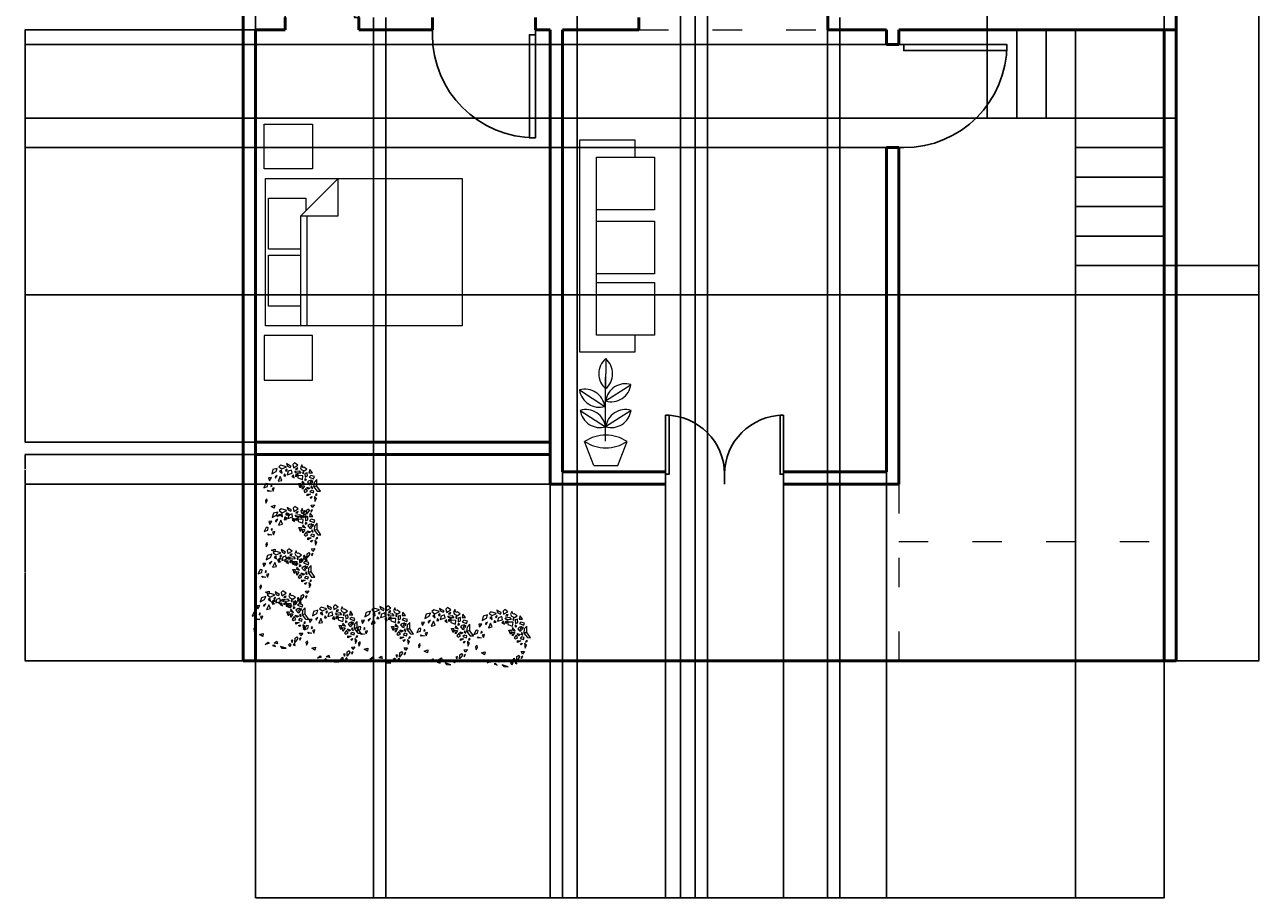
# Model space of a CAD drawing. Units: inches. Extents: x 115999 to 116502, y 188991 to 189729.
# Tile 1 of 5: x 115999 to 116502, y 188991 to 189347. Entities that reach past the tile are written whole.
import ezdxf

# ---------------------------------------------------------------- set-up
doc = ezdxf.new("R2010")
doc.units = ezdxf.units.IN
doc.linetypes.add('ACAD_ISO03W100', pattern=[30, 12, -18])
for name, color, linetype, lineweight in [('A-ANNO-DIMS', 2, 'Continuous', 18), ('A-DOOR', 4, 'Continuous', 25), ('A-FLOR-PRCH', 8, 'ACAD_ISO03W100', 18), ('A-FLOR-STRS', 7, 'Continuous', 25), ('A-FURN', 8, 'Continuous', 18), ('A-WALL', 7, 'Continuous', 50), ('A-WALL-OPEN', 7, 'ACAD_ISO03W100', 18), ('L-PLNT', 3, 'Continuous', 13)]:
    doc.layers.add(name, color=color, linetype=linetype, lineweight=lineweight)
doc.styles.get("Standard").update_dxf_attribs({"font": 'arial.ttf'})
doc.dimstyles.get("Standard").update_dxf_attribs({"dimtxt": 0.18, "dimasz": 0.18, "dimexe": 0.18, "dimexo": 0.0625, "dimgap": 0.09, "dimtad": 0, "dimtih": 1, "dimtoh": 1, "dimdec": 4, "dimzin": 0, "dimdsep": 46, "dimtxsty": 'Standard', "dimcen": 0.09, "dimadec": 0, "dimazin": 0, "dimtfac": 1, "dimtdec": 4, "dimtofl": 0, "dimtmove": 0, "dimatfit": 3, "dimfxl": 1, "dimtolj": 1, "dimtzin": 0, "dimarcsym": 0})

# ---------------------------------------------------------------- blocks, each defined once
blk = doc.blocks.new('*U3')
for p, q in [((0, 0), (0, -5)), ((30, 0), (30, -5))]:
    blk.add_line(p, q)
blk.add_lwpolyline([(0, 0), (0, 30), (1.75, 30), (1.75, 0)], close=True)
blk.add_arc((0, 0), 30, 0, 90)
blk = doc.blocks.new('Bed - Queen')
for p, q in [((0, -80.00003), (0, 0)), ((0, 0), (59.99999, 0)), ((59.99999, 0), (59.99999, -80.00003)), ((7.99999, -1.2), (28.79998, -1.2)), ((7.99999, -14.4), (7.99999, -1.2)), ((28.79998, -1.2), (28.79998, -14.4)), ((31.19999, -1.2), (51.99999, -1.2)), ((31.19999, -14.4), (31.19999, -1.2)), ((51.99999, -1.2), (51.99999, -16.4)), ((0, -14.4), (44.8, -14.4)), ((59.99999, -29.6), (44.8, -14.4)), ((44.8, -14.4), (44.8, -29.6)), ((44.8, -16.8), (0, -16.8)), ((51.99999, -16.4), (46.79936, -16.4)), ((44.8, -29.6), (59.99999, -29.6)), ((59.99999, -80.00003), (0, -80.00003))]:
    blk.add_line(p, q)
blk = doc.blocks.new('*U9')
for points in [[(-4.43, 11.05), (-5.18, 10.36), (-3.96, 9.49), (-2.07, 10.36)], [(-2, 11.66), (-1.6, 10.62), (-0.52, 10.1), (-0.18, 10.62), (-0.79, 10.96)], [(1.24, 12), (0.56, 11.31), (0.76, 10.01), (2.52, 11.05)], [(4.14, 11.14), (3.6, 10.01), (4, 9.23), (5.22, 8.71), (6.3, 9.41), (5.08, 10.19), (4.61, 10.01)], [(-8.14, 6.03), (-9.36, 5.95), (-9.02, 4.73)], [(-5.78, 9.75), (-7.54, 9.23), (-8.01, 7.5), (-6.26, 8.45)], [(-5.78, 6.81), (-6.66, 6.21), (-6.52, 5.69)], [(-4.57, 6.38), (-5.45, 4.47), (-3.89, 4.82)], [(-4.84, 8.63), (-3.83, 7.85), (-4.03, 8.97)], [(-2.88, 7.5), (-3.15, 6.64), (-2.27, 6.72)], [(-1.94, 9.49), (-2.48, 8.97), (-2.27, 8.54), (-1.8, 9.06)], [(0.02, 9.06), (-1.33, 8.54), (-1.73, 7.16), (0.29, 7.76)], [(0.76, 7.16), (0.09, 6.46), (1.1, 5.95)], [(1.37, 8.54), (3.13, 8.8), (3.8, 7.85), (1.91, 7.76)], [(2.59, 9.93), (1.84, 9.75), (1.64, 9.23), (2.32, 9.41)], [(1.71, 6.29), (1.71, 7.07), (2.65, 7.5), (2.11, 6.9)], [(2.52, 6.81), (2.52, 5.86), (4.41, 5.17), (4.61, 6.72)], [(4.61, 8.28), (4.54, 7.76), (4.95, 7.59), (4.95, 8.28)], [(5.49, 5.51), (5.42, 4.82), (6.16, 5.08)], [(6.43, 7.94), (5.49, 7.68), (5.56, 6.21), (6.5, 6.64)], [(7.45, 9.32), (7.11, 7.94), (8.52, 7.94)], [(7.85, 6.81), (7.18, 6.21), (9, 5.51), (9.33, 6.38)], [(10.28, 5.17), (9.2, 4.04), (9, 2.31), (10.48, 0.49), (11.76, 0.41), (10.35, 2.48), (9.33, 2.4), (10.28, 2.83)], [(-11.32, 1.79), (-9.83, 2.31), (-9.63, 3.44), (-10.44, 3.52)], [(-8.21, 0.41), (-9.43, 0.32), (-9.83, 0.84)], [(-8.21, 3.09), (-8.48, 2.31), (-7.87, 2.57)], [(-7, 1.79), (-7.94, 1.53), (-7.47, 0.49)], [(3.53, 1.88), (2.86, 3.52), (3.8, 3.52)], [(4.41, 4.56), (4.27, 3.7), (5.49, 3.26)], [(4.27, 2.74), (5.29, 2.66), (4.41, 1.27)], [(5.83, 1.53), (5.02, 0.41), (5.49, -0.02), (6.5, 0.41)], [(7.51, 1.71), (6.91, 1.27), (6.23, 2.14)], [(8.12, 4.99), (7.11, 4.65), (6.5, 4.13), (7.38, 3.09), (8.12, 3.52), (7.65, 3.87)], [(8.12, 0.75), (7.51, 0.15), (8.93, -0.28), (9.13, 0.49)], [(8.19, 2.57), (7.92, 2.05), (8.66, 1.53)], [(8.73, 4.73), (8.19, 4.56), (8.39, 3.87), (8.59, 4.04)], [(-10.03, -2.71), (-10.64, -3.31), (-10.44, -4.44), (-9.9, -3.49)], [(7.78, -0.8), (6.43, -1.5), (6.43, -0.72)], [(8.32, -1.75), (7.98, -2.53), (7.58, -2.1)], [(9.33, -1.75), (9.54, -3.74), (10.14, -2.53)], [(10.08, -0.63), (9.74, -1.32), (10.48, -0.89)], [(-8.28, -5.73), (-6.79, -5.3), (-7, -6.51)], [(-4.84, -8.85), (-4.43, -9.45), (-5.99, -9.8)], [(-2.34, -9.2), (-1.26, -8.5), (-0.99, -9.54)], [(4.07, -9.45), (3.53, -9.97), (4.07, -10.58), (4.61, -9.89)], [(5.29, -7.98), (4.61, -8.16), (5.02, -8.94)], [(6.03, -9.45), (5.42, -9.97), (6.16, -10.15)], [(6.1, -8.94), (6.16, -7.21), (6.91, -6.69), (7.24, -7.38)], [(8.05, -8.07), (8.59, -7.12), (7.92, -7.55)], [(9.33, -5.13), (8.46, -6.25), (7.98, -5.22)], [(-2.54, -10.06), (-3.02, -10.23), (-1.8, -10.67)], [(0.22, -10.58), (0.83, -11.27), (2.59, -11.36)]]:
    blk.add_lwpolyline(points, close=True)
blk = doc.blocks.new('SOFA-3-SEAT')
for points in [[(22.47, 6.88), (22.47, 0), (0, 0), (0, 86.44), (22.47, 86.44), (22.47, 79.43)], [(29.89, 6.88), (6.84, 6.88), (6.84, 79.43), (29.89, 79.43)]]:
    blk.add_lwpolyline(points)
for points in [[(30.42, 57.99), (6.84, 57.99), (6.84, 79.43), (30.42, 79.43)], [(30.42, 31.86), (6.84, 31.86), (6.84, 53.3), (30.42, 53.3)], [(30.42, 6.88), (6.84, 6.88), (6.84, 28.33), (30.42, 28.33)]]:
    blk.add_lwpolyline(points, close=True)
blk = doc.blocks.new('TABLE-NIGHTSTAND')
blk.add_lwpolyline([(0, 18.2), (19.71, 18.2), (19.71, 0), (0, 0)], close=True)
blk = doc.blocks.new('PLANT-LEAF')
blk.add_line((0, 0.31), (10.34, 7.03))
for centre, start, end in [((8.1, -0.84), 74.1664, 171.9129), ((2.23, 8.18), 254.1664, 351.9129)]:
    blk.add_arc(centre, 8.18, start, end)
blk = doc.blocks.new('*D33')
at = {"layer": 'A-ANNO-DIMS', "color": 0, "lineweight": -2, "transparency": 16777216}
for p, q in [((116088.06, 189088.01), (116088.06, 189728.73)), ((116088.24, 189728.55), (116277.77, 189728.55)), ((116467.88, 189728.55), (116278.35, 189728.55)), ((116468.06, 189088.01), (116468.06, 189728.73))]:
    blk.add_line(p, q, dxfattribs=at)
at = {"layer": 'A-ANNO-DIMS', "color": 0, "transparency": 16777216}
for points in [[(116088.24, 189728.58), (116088.24, 189728.52), (116088.06, 189728.55)], [(116467.88, 189728.58), (116467.88, 189728.52), (116468.06, 189728.55)]]:
    blk.add_solid(points, dxfattribs=at)
at = {"layer": 'Defpoints', "color": 0, "transparency": 16777216}
for p in [(116468.06, 189728.55), (116088.06, 189087.95), (116468.06, 189087.95)]:
    blk.add_point(p, dxfattribs=at)
at = {"layer": 'A-ANNO-DIMS', "color": 0, "transparency": 16777216, "insert": (116278.06, 189728.55), "char_height": 0.18, "attachment_point": 5}
blk.add_mtext('\\A1;380', dxfattribs=at)
blk = doc.blocks.new('*D34')
at = {"layer": 'A-ANNO-DIMS', "color": 0, "lineweight": -2, "transparency": 16777216}
for p, q in [((116468.13, 189694.95), (116501.84, 189694.95)), ((116501.66, 189694.77), (116501.66, 189391.63)), ((116501.66, 189088.13), (116501.66, 189391.27)), ((116468.13, 189087.95), (116501.84, 189087.95))]:
    blk.add_line(p, q, dxfattribs=at)
at = {"layer": 'A-ANNO-DIMS', "color": 0, "transparency": 16777216}
for points in [[(116501.63, 189694.77), (116501.69, 189694.77), (116501.66, 189694.95)], [(116501.63, 189088.13), (116501.69, 189088.13), (116501.66, 189087.95)]]:
    blk.add_solid(points, dxfattribs=at)
at = {"layer": 'Defpoints', "color": 0, "transparency": 16777216}
for p in [(116468.06, 189694.95), (116501.66, 189694.95), (116468.06, 189087.95)]:
    blk.add_point(p, dxfattribs=at)
at = {"layer": 'A-ANNO-DIMS', "color": 0, "transparency": 16777216, "insert": (116501.66, 189391.45), "char_height": 0.18, "attachment_point": 5}
blk.add_mtext('\\A1;607', dxfattribs=at)
blk = doc.blocks.new('*D40')
at = {"layer": 'A-ANNO-DIMS', "color": 0, "lineweight": -2, "transparency": 16777216}
for p, q in [((116093, 189344.95), (115999.04, 189344.95)), ((115999.22, 189344.77), (115999.22, 189261.13)), ((115999.22, 189177.13), (115999.22, 189260.77)), ((116093, 189176.95), (115999.04, 189176.95))]:
    blk.add_line(p, q, dxfattribs=at)
at = {"layer": 'A-ANNO-DIMS', "color": 0, "transparency": 16777216}
for points in [[(115999.19, 189344.77), (115999.25, 189344.77), (115999.22, 189344.95)], [(115999.19, 189177.13), (115999.25, 189177.13), (115999.22, 189176.95)]]:
    blk.add_solid(points, dxfattribs=at)
at = {"layer": 'Defpoints', "color": 0, "transparency": 16777216}
for p in [(116093.06, 189344.95), (115999.22, 189176.95), (116093.06, 189176.95)]:
    blk.add_point(p, dxfattribs=at)
at = {"layer": 'A-ANNO-DIMS', "color": 0, "transparency": 16777216, "insert": (115999.22, 189260.95), "char_height": 0.18, "attachment_point": 5}
blk.add_mtext('\\A1;168', dxfattribs=at)
blk = doc.blocks.new('*D43')
at = {"layer": 'A-ANNO-DIMS', "color": 0, "lineweight": -2, "transparency": 16777216}
for p, q in [((116093.06, 189624.88), (116093.06, 188991.26)), ((116272.06, 189624.88), (116272.06, 188991.26)), ((116093.24, 188991.44), (116182.28, 188991.44)), ((116271.88, 188991.44), (116182.84, 188991.44))]:
    blk.add_line(p, q, dxfattribs=at)
at = {"layer": 'A-ANNO-DIMS', "color": 0, "transparency": 16777216}
for points in [[(116093.24, 188991.47), (116093.24, 188991.41), (116093.06, 188991.44)], [(116271.88, 188991.47), (116271.88, 188991.41), (116272.06, 188991.44)]]:
    blk.add_solid(points, dxfattribs=at)
at = {"layer": 'Defpoints', "color": 0, "transparency": 16777216}
for p in [(116093.06, 189624.95), (116272.06, 189624.95), (116272.06, 188991.44)]:
    blk.add_point(p, dxfattribs=at)
at = {"layer": 'A-ANNO-DIMS', "color": 0, "transparency": 16777216, "insert": (116182.56, 188991.44), "char_height": 0.18, "attachment_point": 5}
blk.add_mtext('\\A1;179', dxfattribs=at)
blk = doc.blocks.new('*D44')
at = {"layer": 'A-ANNO-DIMS', "color": 0, "lineweight": -2, "transparency": 16777216}
for p, q in [((116277.06, 189624.88), (116277.06, 188991.26)), ((116463.06, 189624.88), (116463.06, 188991.26)), ((116277.24, 188991.44), (116369.78, 188991.44)), ((116462.88, 188991.44), (116370.34, 188991.44))]:
    blk.add_line(p, q, dxfattribs=at)
at = {"layer": 'A-ANNO-DIMS', "color": 0, "transparency": 16777216}
for points in [[(116277.24, 188991.47), (116277.24, 188991.41), (116277.06, 188991.44)], [(116462.88, 188991.47), (116462.88, 188991.41), (116463.06, 188991.44)]]:
    blk.add_solid(points, dxfattribs=at)
at = {"layer": 'Defpoints', "color": 0, "transparency": 16777216}
for p in [(116277.06, 189624.95), (116463.06, 189624.95), (116463.06, 188991.44)]:
    blk.add_point(p, dxfattribs=at)
at = {"layer": 'A-ANNO-DIMS', "color": 0, "transparency": 16777216, "insert": (116370.06, 188991.44), "char_height": 0.18, "attachment_point": 5}
blk.add_mtext('\\A1;186', dxfattribs=at)
blk = doc.blocks.new('*D45')
at = {"layer": 'A-ANNO-DIMS', "color": 0, "lineweight": -2, "transparency": 16777216}
for p, q in [((116272.06, 189624.88), (116272.06, 188991.26)), ((116277.06, 189624.88), (116277.06, 188991.26)), ((116272.24, 188991.44), (116274.41, 188991.44)), ((116276.88, 188991.44), (116274.71, 188991.44))]:
    blk.add_line(p, q, dxfattribs=at)
at = {"layer": 'A-ANNO-DIMS', "color": 0, "transparency": 16777216}
for points in [[(116272.24, 188991.47), (116272.24, 188991.41), (116272.06, 188991.44)], [(116276.88, 188991.47), (116276.88, 188991.41), (116277.06, 188991.44)]]:
    blk.add_solid(points, dxfattribs=at)
at = {"layer": 'Defpoints', "color": 0, "transparency": 16777216}
for p in [(116272.06, 189624.95), (116277.06, 189624.95), (116277.06, 188991.44)]:
    blk.add_point(p, dxfattribs=at)
at = {"layer": 'A-ANNO-DIMS', "color": 0, "transparency": 16777216, "insert": (116274.56, 188991.44), "char_height": 0.18, "attachment_point": 5}
blk.add_mtext('\\A1;5', dxfattribs=at)
blk = doc.blocks.new('*D46')
at = {"layer": 'A-ANNO-DIMS', "color": 0, "lineweight": -2, "transparency": 16777216}
for p, q in [((116224.06, 189486.88), (116224.06, 188991.26)), ((116266.06, 189486.88), (116266.06, 188991.26)), ((116224.24, 188991.44), (116244.84, 188991.44)), ((116265.88, 188991.44), (116245.28, 188991.44))]:
    blk.add_line(p, q, dxfattribs=at)
at = {"layer": 'A-ANNO-DIMS', "color": 0, "transparency": 16777216}
for points in [[(116224.24, 188991.47), (116224.24, 188991.41), (116224.06, 188991.44)], [(116265.88, 188991.47), (116265.88, 188991.41), (116266.06, 188991.44)]]:
    blk.add_solid(points, dxfattribs=at)
at = {"layer": 'Defpoints', "color": 0, "transparency": 16777216}
for p in [(116224.06, 189486.95), (116266.06, 189486.95), (116266.06, 188991.44)]:
    blk.add_point(p, dxfattribs=at)
at = {"layer": 'A-ANNO-DIMS', "color": 0, "transparency": 16777216, "insert": (116245.06, 188991.44), "char_height": 0.18, "attachment_point": 5}
blk.add_mtext('\\A1;42', dxfattribs=at)
blk = doc.blocks.new('*D47')
at = {"layer": 'A-ANNO-DIMS', "color": 0, "lineweight": -2, "transparency": 16777216}
for p, q in [((116266.063078, 189486.884428), (116266.063078, 188991.259265)), ((116272.063078, 189486.884428), (116272.063078, 188991.259265)), ((116266.243078, 188991.439265), (116268.913651, 188991.439265)), ((116271.883078, 188991.439265), (116269.212505, 188991.439265))]:
    blk.add_line(p, q, dxfattribs=at)
at = {"layer": 'A-ANNO-DIMS', "color": 0, "transparency": 16777216}
for points in [[(116266.243078, 188991.469265), (116266.243078, 188991.409265), (116266.063078, 188991.439265)], [(116271.883078, 188991.469265), (116271.883078, 188991.409265), (116272.063078, 188991.439265)]]:
    blk.add_solid(points, dxfattribs=at)
at = {"layer": 'Defpoints', "color": 0, "transparency": 16777216}
for p in [(116266.063078, 189486.946928), (116272.063078, 189486.946928), (116272.063078, 188991.439265)]:
    blk.add_point(p, dxfattribs=at)
at = {"layer": 'A-ANNO-DIMS', "color": 0, "transparency": 16777216, "insert": (116269.063078, 188991.439265), "char_height": 0.18, "attachment_point": 5}
blk.add_mtext('\\A1;6', dxfattribs=at)
blk = doc.blocks.new('*D49')
at = {"layer": 'A-ANNO-DIMS', "color": 0, "lineweight": -2, "transparency": 16777216}
for p, q in [((116331.06, 189349.88), (116331.06, 188991.26)), ((116463.06, 189349.88), (116463.06, 188991.26)), ((116331.24, 188991.44), (116396.78, 188991.44)), ((116462.88, 188991.44), (116397.34, 188991.44))]:
    blk.add_line(p, q, dxfattribs=at)
at = {"layer": 'A-ANNO-DIMS', "color": 0, "transparency": 16777216}
for points in [[(116331.24, 188991.47), (116331.24, 188991.41), (116331.06, 188991.44)], [(116462.88, 188991.47), (116462.88, 188991.41), (116463.06, 188991.44)]]:
    blk.add_solid(points, dxfattribs=at)
at = {"layer": 'Defpoints', "color": 0, "transparency": 16777216}
for p in [(116331.06, 189349.95), (116463.06, 189349.95), (116463.06, 188991.44)]:
    blk.add_point(p, dxfattribs=at)
at = {"layer": 'A-ANNO-DIMS', "color": 0, "transparency": 16777216, "insert": (116397.06, 188991.44), "char_height": 0.18, "attachment_point": 5}
blk.add_mtext('\\A1;132', dxfattribs=at)
blk = doc.blocks.new('*D50')
at = {"layer": 'A-ANNO-DIMS', "color": 0, "lineweight": -2, "transparency": 16777216}
for p, q in [((116146.06, 189349.88), (116146.06, 188991.26)), ((116326.06, 189349.88), (116326.06, 188991.26)), ((116146.24, 188991.44), (116235.78, 188991.44)), ((116325.88, 188991.44), (116236.34, 188991.44))]:
    blk.add_line(p, q, dxfattribs=at)
at = {"layer": 'A-ANNO-DIMS', "color": 0, "transparency": 16777216}
for points in [[(116146.24, 188991.47), (116146.24, 188991.41), (116146.06, 188991.44)], [(116325.88, 188991.47), (116325.88, 188991.41), (116326.06, 188991.44)]]:
    blk.add_solid(points, dxfattribs=at)
at = {"layer": 'Defpoints', "color": 0, "transparency": 16777216}
for p in [(116146.06, 189349.95), (116326.06, 189349.95), (116326.06, 188991.44)]:
    blk.add_point(p, dxfattribs=at)
at = {"layer": 'A-ANNO-DIMS', "color": 0, "transparency": 16777216, "insert": (116236.06, 188991.44), "char_height": 0.18, "attachment_point": 5}
blk.add_mtext('\\A1;180', dxfattribs=at)
blk = doc.blocks.new('*D51')
at = {"layer": 'A-ANNO-DIMS', "color": 0, "lineweight": -2, "transparency": 16777216}
for p, q in [((116093.06, 189349.88), (116093.06, 188991.26)), ((116141.06, 189349.88), (116141.06, 188991.26)), ((116093.24, 188991.44), (116116.84, 188991.44)), ((116140.88, 188991.44), (116117.29, 188991.44))]:
    blk.add_line(p, q, dxfattribs=at)
at = {"layer": 'A-ANNO-DIMS', "color": 0, "transparency": 16777216}
for points in [[(116093.24, 188991.47), (116093.24, 188991.41), (116093.06, 188991.44)], [(116140.88, 188991.47), (116140.88, 188991.41), (116141.06, 188991.44)]]:
    blk.add_solid(points, dxfattribs=at)
at = {"layer": 'Defpoints', "color": 0, "transparency": 16777216}
for p in [(116093.06, 189349.95), (116141.06, 189349.95), (116141.06, 188991.44)]:
    blk.add_point(p, dxfattribs=at)
at = {"layer": 'A-ANNO-DIMS', "color": 0, "transparency": 16777216, "insert": (116117.06, 188991.44), "char_height": 0.18, "attachment_point": 5}
blk.add_mtext('\\A1;48', dxfattribs=at)
blk = doc.blocks.new('*D56')
at = {"layer": 'A-ANNO-DIMS', "color": 0, "lineweight": -2, "transparency": 16777216}
for p, q in [((116093.06, 189176.88), (116093.06, 188991.26)), ((116213.06, 189176.88), (116213.06, 188991.26)), ((116093.24, 188991.44), (116152.78, 188991.44)), ((116212.88, 188991.44), (116153.34, 188991.44))]:
    blk.add_line(p, q, dxfattribs=at)
at = {"layer": 'A-ANNO-DIMS', "color": 0, "transparency": 16777216}
for points in [[(116093.24, 188991.47), (116093.24, 188991.41), (116093.06, 188991.44)], [(116212.88, 188991.47), (116212.88, 188991.41), (116213.06, 188991.44)]]:
    blk.add_solid(points, dxfattribs=at)
at = {"layer": 'Defpoints', "color": 0, "transparency": 16777216}
for p in [(116093.06, 189176.95), (116213.06, 189176.95), (116213.06, 188991.44)]:
    blk.add_point(p, dxfattribs=at)
at = {"layer": 'A-ANNO-DIMS', "color": 0, "transparency": 16777216, "insert": (116153.06, 188991.44), "char_height": 0.18, "attachment_point": 5}
blk.add_mtext('\\A1;120', dxfattribs=at)
blk = doc.blocks.new('*D57')
at = {"layer": 'A-ANNO-DIMS', "color": 0, "lineweight": -2, "transparency": 16777216}
for p, q in [((116218.06, 189164.88), (116218.06, 188991.26)), ((116260.06, 189164.88), (116260.06, 188991.26)), ((116218.24, 188991.44), (116238.84, 188991.44)), ((116259.88, 188991.44), (116239.28, 188991.44))]:
    blk.add_line(p, q, dxfattribs=at)
at = {"layer": 'A-ANNO-DIMS', "color": 0, "transparency": 16777216}
for points in [[(116218.24, 188991.47), (116218.24, 188991.41), (116218.06, 188991.44)], [(116259.88, 188991.47), (116259.88, 188991.41), (116260.06, 188991.44)]]:
    blk.add_solid(points, dxfattribs=at)
at = {"layer": 'Defpoints', "color": 0, "transparency": 16777216}
for p in [(116218.06, 189164.95), (116260.06, 189164.95), (116260.06, 188991.44)]:
    blk.add_point(p, dxfattribs=at)
at = {"layer": 'A-ANNO-DIMS', "color": 0, "transparency": 16777216, "insert": (116239.06, 188991.44), "char_height": 0.18, "attachment_point": 5}
blk.add_mtext('\\A1;42', dxfattribs=at)
blk = doc.blocks.new('*D58')
at = {"layer": 'A-ANNO-DIMS', "color": 0, "lineweight": -2, "transparency": 16777216}
for p, q in [((116260.06, 189164.88), (116260.06, 188991.26)), ((116308.06, 189164.88), (116308.06, 188991.26)), ((116260.24, 188991.44), (116283.84, 188991.44)), ((116307.88, 188991.44), (116284.29, 188991.44))]:
    blk.add_line(p, q, dxfattribs=at)
at = {"layer": 'A-ANNO-DIMS', "color": 0, "transparency": 16777216}
for points in [[(116260.24, 188991.47), (116260.24, 188991.41), (116260.06, 188991.44)], [(116307.88, 188991.47), (116307.88, 188991.41), (116308.06, 188991.44)]]:
    blk.add_solid(points, dxfattribs=at)
at = {"layer": 'Defpoints', "color": 0, "transparency": 16777216}
for p in [(116260.06, 189164.95), (116308.06, 189164.95), (116308.06, 188991.44)]:
    blk.add_point(p, dxfattribs=at)
at = {"layer": 'A-ANNO-DIMS', "color": 0, "transparency": 16777216, "insert": (116284.06, 188991.44), "char_height": 0.18, "attachment_point": 5}
blk.add_mtext('\\A1;48', dxfattribs=at)
blk = doc.blocks.new('*D59')
at = {"layer": 'A-ANNO-DIMS', "color": 0, "lineweight": -2, "transparency": 16777216}
for p, q in [((116308.06, 189164.88), (116308.06, 188991.26)), ((116350.06, 189164.88), (116350.06, 188991.26)), ((116308.24, 188991.44), (116328.84, 188991.44)), ((116349.88, 188991.44), (116329.28, 188991.44))]:
    blk.add_line(p, q, dxfattribs=at)
at = {"layer": 'A-ANNO-DIMS', "color": 0, "transparency": 16777216}
for points in [[(116308.24, 188991.47), (116308.24, 188991.41), (116308.06, 188991.44)], [(116349.88, 188991.47), (116349.88, 188991.41), (116350.06, 188991.44)]]:
    blk.add_solid(points, dxfattribs=at)
at = {"layer": 'Defpoints', "color": 0, "transparency": 16777216}
for p in [(116308.06, 189164.95), (116350.06, 189164.95), (116350.06, 188991.44)]:
    blk.add_point(p, dxfattribs=at)
at = {"layer": 'A-ANNO-DIMS', "color": 0, "transparency": 16777216, "insert": (116329.06, 188991.44), "char_height": 0.18, "attachment_point": 5}
blk.add_mtext('\\A1;42', dxfattribs=at)
blk = doc.blocks.new('*D60')
at = {"layer": 'A-ANNO-DIMS', "color": 0, "lineweight": -2, "transparency": 16777216}
for p, q in [((116213, 189159.95), (115999.04, 189159.95)), ((115999.22, 189159.77), (115999.22, 189124.13)), ((115999.22, 189088.13), (115999.22, 189123.77)), ((116088, 189087.95), (115999.04, 189087.95))]:
    blk.add_line(p, q, dxfattribs=at)
at = {"layer": 'A-ANNO-DIMS', "color": 0, "transparency": 16777216}
for points in [[(115999.19, 189159.77), (115999.25, 189159.77), (115999.22, 189159.95)], [(115999.19, 189088.13), (115999.25, 189088.13), (115999.22, 189087.95)]]:
    blk.add_solid(points, dxfattribs=at)
at = {"layer": 'Defpoints', "color": 0, "transparency": 16777216}
for p in [(116213.06, 189159.95), (115999.22, 189087.95), (116088.06, 189087.95)]:
    blk.add_point(p, dxfattribs=at)
at = {"layer": 'A-ANNO-DIMS', "color": 0, "transparency": 16777216, "insert": (115999.22, 189123.95), "char_height": 0.18, "attachment_point": 5}
blk.add_mtext('\\A1;72', dxfattribs=at)
blk = doc.blocks.new('*D61')
at = {"layer": 'A-ANNO-DIMS', "color": 0, "lineweight": -2, "transparency": 16777216}
for p, q in [((116213, 189171.95), (115999.04, 189171.95)), ((115999.22, 189171.77), (115999.22, 189166.13)), ((115999.22, 189160.13), (115999.22, 189165.77)), ((116213, 189159.95), (115999.04, 189159.95))]:
    blk.add_line(p, q, dxfattribs=at)
at = {"layer": 'A-ANNO-DIMS', "color": 0, "transparency": 16777216}
for points in [[(115999.19, 189171.77), (115999.25, 189171.77), (115999.22, 189171.95)], [(115999.19, 189160.13), (115999.25, 189160.13), (115999.22, 189159.95)]]:
    blk.add_solid(points, dxfattribs=at)
at = {"layer": 'Defpoints', "color": 0, "transparency": 16777216}
for p in [(116213.06, 189171.95), (115999.22, 189159.95), (116213.06, 189159.95)]:
    blk.add_point(p, dxfattribs=at)
at = {"layer": 'A-ANNO-DIMS', "color": 0, "transparency": 16777216, "insert": (115999.22, 189165.95), "char_height": 0.18, "attachment_point": 5}
blk.add_mtext('\\A1;12', dxfattribs=at)
blk = doc.blocks.new('*D62')
at = {"layer": 'A-ANNO-DIMS', "color": 0, "lineweight": -2, "transparency": 16777216}
for p, q in [((116427.06, 189236.88), (116427.06, 188991.26)), ((116463.06, 189236.88), (116463.06, 188991.26)), ((116427.24, 188991.44), (116444.84, 188991.44)), ((116462.88, 188991.44), (116445.28, 188991.44))]:
    blk.add_line(p, q, dxfattribs=at)
at = {"layer": 'A-ANNO-DIMS', "color": 0, "transparency": 16777216}
for points in [[(116427.24, 188991.47), (116427.24, 188991.41), (116427.06, 188991.44)], [(116462.88, 188991.47), (116462.88, 188991.41), (116463.06, 188991.44)]]:
    blk.add_solid(points, dxfattribs=at)
at = {"layer": 'Defpoints', "color": 0, "transparency": 16777216}
for p in [(116427.06, 189236.95), (116463.06, 189236.95), (116463.06, 188991.44)]:
    blk.add_point(p, dxfattribs=at)
at = {"layer": 'A-ANNO-DIMS', "color": 0, "transparency": 16777216, "insert": (116445.06, 188991.44), "char_height": 0.18, "attachment_point": 5}
blk.add_mtext('\\A1;36', dxfattribs=at)
blk = doc.blocks.new('*D63')
at = {"layer": 'A-ANNO-DIMS', "color": 0, "lineweight": -2, "transparency": 16777216}
for p, q in [((116415, 189308.95), (115999.04, 189308.95)), ((115999.22, 189308.77), (115999.22, 189273.13)), ((115999.22, 189237.13), (115999.22, 189272.77)), ((116427, 189236.95), (115999.04, 189236.95))]:
    blk.add_line(p, q, dxfattribs=at)
at = {"layer": 'A-ANNO-DIMS', "color": 0, "transparency": 16777216}
for points in [[(115999.19, 189308.77), (115999.25, 189308.77), (115999.22, 189308.95)], [(115999.19, 189237.13), (115999.25, 189237.13), (115999.22, 189236.95)]]:
    blk.add_solid(points, dxfattribs=at)
at = {"layer": 'Defpoints', "color": 0, "transparency": 16777216}
for p in [(116415.06, 189308.95), (115999.22, 189236.95), (116427.06, 189236.95)]:
    blk.add_point(p, dxfattribs=at)
at = {"layer": 'A-ANNO-DIMS', "color": 0, "transparency": 16777216, "insert": (115999.22, 189272.95), "char_height": 0.18, "attachment_point": 5}
blk.add_mtext('\\A1;72', dxfattribs=at)
blk = doc.blocks.new('*D64')
at = {"layer": 'A-ANNO-DIMS', "color": 0, "lineweight": -2, "transparency": 16777216}
for p, q in [((116463.13, 189248.95), (116501.84, 189248.95)), ((116501.66, 189248.77), (116501.66, 189243.13)), ((116501.66, 189237.13), (116501.66, 189242.77)), ((116463.13, 189236.95), (116501.84, 189236.95))]:
    blk.add_line(p, q, dxfattribs=at)
at = {"layer": 'A-ANNO-DIMS', "color": 0, "transparency": 16777216}
for points in [[(116501.63, 189248.77), (116501.69, 189248.77), (116501.66, 189248.95)], [(116501.63, 189237.13), (116501.69, 189237.13), (116501.66, 189236.95)]]:
    blk.add_solid(points, dxfattribs=at)
at = {"layer": 'Defpoints', "color": 0, "transparency": 16777216}
for p in [(116463.06, 189248.95), (116463.06, 189236.95), (116501.66, 189236.95)]:
    blk.add_point(p, dxfattribs=at)
at = {"layer": 'A-ANNO-DIMS', "color": 0, "transparency": 16777216, "insert": (116501.66, 189242.95), "char_height": 0.18, "attachment_point": 5}
blk.add_mtext('\\A1;12', dxfattribs=at)
blk = doc.blocks.new('*D65')
at = {"layer": 'A-ANNO-DIMS', "color": 0, "lineweight": -2, "transparency": 16777216}
for p, q in [((116391.06, 189309.01), (116391.06, 189728.73)), ((116391.24, 189728.55), (116426.85, 189728.55)), ((116462.88, 189728.55), (116427.28, 189728.55)), ((116463.06, 189237.01), (116463.06, 189728.73))]:
    blk.add_line(p, q, dxfattribs=at)
at = {"layer": 'A-ANNO-DIMS', "color": 0, "transparency": 16777216}
for points in [[(116391.24, 189728.58), (116391.24, 189728.52), (116391.06, 189728.55)], [(116462.88, 189728.58), (116462.88, 189728.52), (116463.06, 189728.55)]]:
    blk.add_solid(points, dxfattribs=at)
at = {"layer": 'Defpoints', "color": 0, "transparency": 16777216}
for p in [(116463.06, 189728.55), (116391.06, 189308.95), (116463.06, 189236.95)]:
    blk.add_point(p, dxfattribs=at)
at = {"layer": 'A-ANNO-DIMS', "color": 0, "transparency": 16777216, "insert": (116427.06, 189728.55), "char_height": 0.18, "attachment_point": 5}
blk.add_mtext('\\A1;72', dxfattribs=at)
blk = doc.blocks.new('*D66')
at = {"layer": 'A-ANNO-DIMS', "color": 0, "lineweight": -2, "transparency": 16777216}
for p, q in [((116355, 189338.95), (115999.04, 189338.95)), ((115999.22, 189338.77), (115999.22, 189318.13)), ((115999.22, 189297.13), (115999.22, 189317.77)), ((116355, 189296.95), (115999.04, 189296.95))]:
    blk.add_line(p, q, dxfattribs=at)
at = {"layer": 'A-ANNO-DIMS', "color": 0, "transparency": 16777216}
for points in [[(115999.19, 189338.77), (115999.25, 189338.77), (115999.22, 189338.95)], [(115999.19, 189297.13), (115999.25, 189297.13), (115999.22, 189296.95)]]:
    blk.add_solid(points, dxfattribs=at)
at = {"layer": 'Defpoints', "color": 0, "transparency": 16777216}
for p in [(115999.22, 189338.95), (116355.06, 189338.95), (116355.06, 189296.95)]:
    blk.add_point(p, dxfattribs=at)
at = {"layer": 'A-ANNO-DIMS', "color": 0, "transparency": 16777216, "insert": (115999.22, 189317.95), "char_height": 0.18, "attachment_point": 5}
blk.add_mtext('\\A1;42', dxfattribs=at)

msp = doc.modelspace()

# ---------------------------------------------------------------- linework, layer by layer
at = {"layer": 'A-FLOR-PRCH'}
for p, q in [((116213.0631, 189159.9469), (116213.0631, 189087.9469)), ((116355.0631, 189159.9469), (116355.0631, 189087.9469)), ((116355.0631, 189136.528), (116463.0631, 189136.528))]:
    msp.add_line(p, q, dxfattribs=at)
at = {"layer": 'A-FLOR-STRS'}
for p, q in [((116391.0631, 189344.9469), (116391.0631, 189308.9469)), ((116403.0631, 189344.9469), (116403.0631, 189308.9469)), ((116415.0631, 189344.9469), (116415.0631, 189308.9469)), ((116427.0631, 189344.9469), (116427.0631, 189236.9469)), ((116391.0631, 189308.9469), (116468.0631, 189308.9469)), ((116427.0631, 189296.9469), (116463.0631, 189296.9469)), ((116427.0631, 189284.9469), (116463.0631, 189284.9469)), ((116427.0631, 189272.9469), (116463.0631, 189272.9469)), ((116427.0631, 189260.9469), (116463.0631, 189260.9469)), ((116427.0631, 189248.9469), (116463.0631, 189248.9469)), ((116427.0631, 189236.9469), (116463.0631, 189236.9469))]:
    msp.add_line(p, q, dxfattribs=at)
at = {"layer": 'A-WALL'}
for p, q in [((116088.0631, 189694.9469), (116088.0631, 189087.9469)), ((116468.0631, 189694.9469), (116468.0631, 189087.9469)), ((116326.0631, 189392.6745), (116326.0631, 189344.9469)), ((116105.0631, 189349.9469), (116105.0631, 189344.9469)), ((116135.0631, 189349.9469), (116135.0631, 189344.9469)), ((116165.0631, 189344.9469), (116165.0631, 189349.9469)), ((116207.0631, 189344.9469), (116207.0631, 189349.9469)), ((116249.1823, 189344.9469), (116249.1823, 189349.9469)), ((116093.0631, 189344.9469), (116105.0631, 189344.9469)), ((116093.0631, 189344.9469), (116093.0631, 189087.9469)), ((116135.0631, 189344.9469), (116165.0631, 189344.9469)), ((116207.0631, 189344.9469), (116213.0631, 189344.9469)), ((116213.0631, 189344.9469), (116213.0631, 189159.9469)), ((116218.0631, 189344.9469), (116218.0631, 189164.9469)), ((116218.0631, 189344.9469), (116249.1823, 189344.9469)), ((116326.0631, 189344.9469), (116350.0631, 189344.9469)), ((116350.0631, 189344.9469), (116350.0631, 189338.9469)), ((116355.0631, 189344.9469), (116355.0631, 189338.9469)), ((116355.0631, 189344.9469), (116468.0631, 189344.9469)), ((116463.0631, 189344.9469), (116463.0631, 189087.9469)), ((116355.0631, 189338.9469), (116350.0631, 189338.9469)), ((116355.0631, 189296.9469), (116350.0631, 189296.9469)), ((116350.0631, 189296.9469), (116350.0631, 189164.9469)), ((116355.0631, 189296.9469), (116355.0631, 189159.9469)), ((116093.0631, 189176.9469), (116213.0631, 189176.9469)), ((116093.0631, 189171.9469), (116213.0631, 189171.9469)), ((116218.0631, 189164.9469), (116260.0631, 189164.9469)), ((116308.0631, 189164.9469), (116350.0631, 189164.9469)), ((116213.0631, 189159.9469), (116260.0631, 189159.9469)), ((116308.0631, 189159.9469), (116355.0631, 189159.9469)), ((116088.0631, 189087.9469), (116468.0631, 189087.9469))]:
    msp.add_line(p, q, dxfattribs=at)
at = {"layer": 'A-WALL-OPEN'}
for p, q in [((116249.1823, 189344.9469), (116326.0631, 189344.9469)), ((116260.0631, 189164.9469), (116260.0631, 189159.9469)), ((116308.0631, 189164.9469), (116308.0631, 189159.9469))]:
    msp.add_line(p, q, dxfattribs=at)
at = {"layer": 'L-PLNT'}
for p, q in [((116235.6278, 189177.3571), (116235.6278, 189203.4158)), ((116230.8305, 189167.5382), (116227.075, 189177.2814)), ((116240.5931, 189167.5382), (116244.3486, 189177.2814)), ((116230.8305, 189167.5382), (116240.5931, 189167.5382))]:
    msp.add_line(p, q, dxfattribs=at)
for centre, start, end in [((116235.7118, 189164.2138), 56.53812, 123.46188), ((116235.7118, 189190.3491), 236.53812, 303.46188)]:
    msp.add_arc(centre, 15.6639, start, end, dxfattribs=at)

# ---------------------------------------------------------------- block references
at = {"layer": 'A-DOOR', "xscale": -1}
msp.add_blockref('*U3', (116135.0631, 189349.9469), dxfattribs=at)
at = {"layer": 'A-DOOR', "xscale": 1.400000000000193, "yscale": 1.400000000000193, "zscale": 1.400000000000193}
for p, rotation in [((116207.0631, 189342.9469), 180), ((116357.0631, 189338.9469), 270)]:
    msp.add_blockref('*U3', p, dxfattribs=dict(at, rotation=rotation))
at = {"layer": 'A-DOOR', "yscale": 0.8000000000002424, "zscale": 0.8000000000002424}
for p, xscale in [((116260.0631, 189163.9469), 0.8000000000002424), ((116308.0631, 189163.9469), -0.8000000000002424)]:
    msp.add_blockref('*U3', p, dxfattribs=dict(at, xscale=xscale))
at = {"layer": 'A-FURN'}
for name, p in [('TABLE-NIGHTSTAND', (116096.5803, 189288.2647)), ('SOFA-3-SEAT', (116225.0717, 189213.6836))]:
    msp.add_blockref(name, p, dxfattribs=at)
at = {"layer": 'A-FURN', "rotation": 90}
msp.add_blockref('Bed - Queen', (116097.142, 189224.3647), dxfattribs=at)
at = {"layer": 'A-FURN', "extrusion": (0, 0, -1), "zscale": -1, "rotation": 180}
msp.add_blockref('TABLE-NIGHTSTAND', (-116096.5803, 189220.4647), dxfattribs=at)
at = {"layer": 'L-PLNT'}
for p, rotation in [((116235.4025, 189211.2175), 236.8009428572069), ((116224.7176, 189198.132), 293.920701119743), ((116225.008, 189189.8444), 293.9207011199753), ((116245.964, 189190.2804), 180)]:
    msp.add_blockref('PLANT-LEAF', p, dxfattribs=dict(at, rotation=rotation))
for name, p in [('PLANT-LEAF', (116235.628, 189193.471)), ('*U9', (116107.6901, 189156.5945)), ('*U9', (116107.8704, 189138.7999)), ('*U9', (116105.4187, 189121.6112)), ('*U9', (116102.9671, 189104.4225)), ('*U9', (116124.2129, 189098.8027)), ('*U9', (116145.6179, 189098.4271)), ('*U9', (116170.0265, 189097.6769)), ('*U9', (116193.3094, 189096.9263))]:
    msp.add_blockref(name, p, dxfattribs=at)

# ---------------------------------------------------------------- dimensions: what is measured, and where the dimension line sits
at = {"layer": 'A-ANNO-DIMS'}
for base, p1, p2, picture, middle in [((116468.0631, 189728.5469), (116088.0631, 189087.9469), (116468.0631, 189087.9469), '*D33', (116278.0631, 189728.5469)), ((116463.0631, 189728.5469), (116391.0631, 189308.9469), (116463.0631, 189236.9469), '*D65', (116427.0631, 189728.5469)), ((116272.0631, 188991.4393), (116093.0631, 189624.9469), (116272.0631, 189624.9469), '*D43', (116182.5631, 188991.4393)), ((116277.0631, 188991.4393), (116272.0631, 189624.9469), (116277.0631, 189624.9469), '*D45', (116274.5631, 188991.4393)), ((116463.0631, 188991.4393), (116277.0631, 189624.9469), (116463.0631, 189624.9469), '*D44', (116370.0631, 188991.4393)), ((116266.0631, 188991.4393), (116224.0631, 189486.9469), (116266.0631, 189486.9469), '*D46', (116245.0631, 188991.4393)), ((116272.0631, 188991.4393), (116266.0631, 189486.9469), (116272.0631, 189486.9469), '*D47', (116269.0631, 188991.4393)), ((116141.0631, 188991.4393), (116093.0631, 189349.9469), (116141.0631, 189349.9469), '*D51', (116117.0631, 188991.4393)), ((116326.0631, 188991.4393), (116146.0631, 189349.9469), (116326.0631, 189349.9469), '*D50', (116236.0631, 188991.4393)), ((116463.0631, 188991.4393), (116331.0631, 189349.9469), (116463.0631, 189349.9469), '*D49', (116397.0631, 188991.4393)), ((116463.0631, 188991.4393), (116427.0631, 189236.9469), (116463.0631, 189236.9469), '*D62', (116445.0631, 188991.4393)), ((116213.0631, 188991.4393), (116093.0631, 189176.9469), (116213.0631, 189176.9469), '*D56', (116153.0631, 188991.4393)), ((116260.0631, 188991.4393), (116218.0631, 189164.9469), (116260.0631, 189164.9469), '*D57', (116239.0631, 188991.4393)), ((116308.0631, 188991.4393), (116260.0631, 189164.9469), (116308.0631, 189164.9469), '*D58', (116284.0631, 188991.4393)), ((116350.0631, 188991.4393), (116308.0631, 189164.9469), (116350.0631, 189164.9469), '*D59', (116329.0631, 188991.4393))]:
    dim = msp.add_linear_dim(base=base, p1=p1, p2=p2, dimstyle='Standard', override={"dimdec": 0, "dimlfac": 1, "dimrnd": 0, "dimzin": 0, "dimdsep": 46, "dimlunit": 2}, dxfattribs=at)
    dim.commit()
    dim.dimension.update_dxf_attribs({"geometry": picture, "text_midpoint": middle})
for base, p1, p2, picture, middle in [((116501.6631, 189694.9469), (116468.0631, 189087.9469), (116468.0631, 189694.9469), '*D34', (116501.6631, 189391.4469)), ((115999.2211, 189176.9469), (116093.0631, 189344.9469), (116093.0631, 189176.9469), '*D40', (115999.2211, 189260.9469)), ((115999.2211, 189338.9469), (116355.0631, 189296.9469), (116355.0631, 189338.9469), '*D66', (115999.2211, 189317.9469)), ((115999.2211, 189236.9469), (116415.0631, 189308.9469), (116427.0631, 189236.9469), '*D63', (115999.2211, 189272.9469)), ((116501.6631, 189236.9469), (116463.0631, 189248.9469), (116463.0631, 189236.9469), '*D64', (116501.6631, 189242.9469)), ((115999.2211, 189159.9469), (116213.0631, 189171.9469), (116213.0631, 189159.9469), '*D61', (115999.2211, 189165.9469)), ((115999.2211, 189087.9469), (116213.0631, 189159.9469), (116088.0631, 189087.9469), '*D60', (115999.2211, 189123.9469))]:
    dim = msp.add_linear_dim(base=base, p1=p1, p2=p2, angle=90, dimstyle='Standard', override={"dimdec": 0, "dimlfac": 1, "dimrnd": 0, "dimzin": 0, "dimdsep": 46, "dimlunit": 2}, dxfattribs=at)
    dim.commit()
    dim.dimension.update_dxf_attribs({"geometry": picture, "text_midpoint": middle})

doc.saveas('drawing.dxf')
